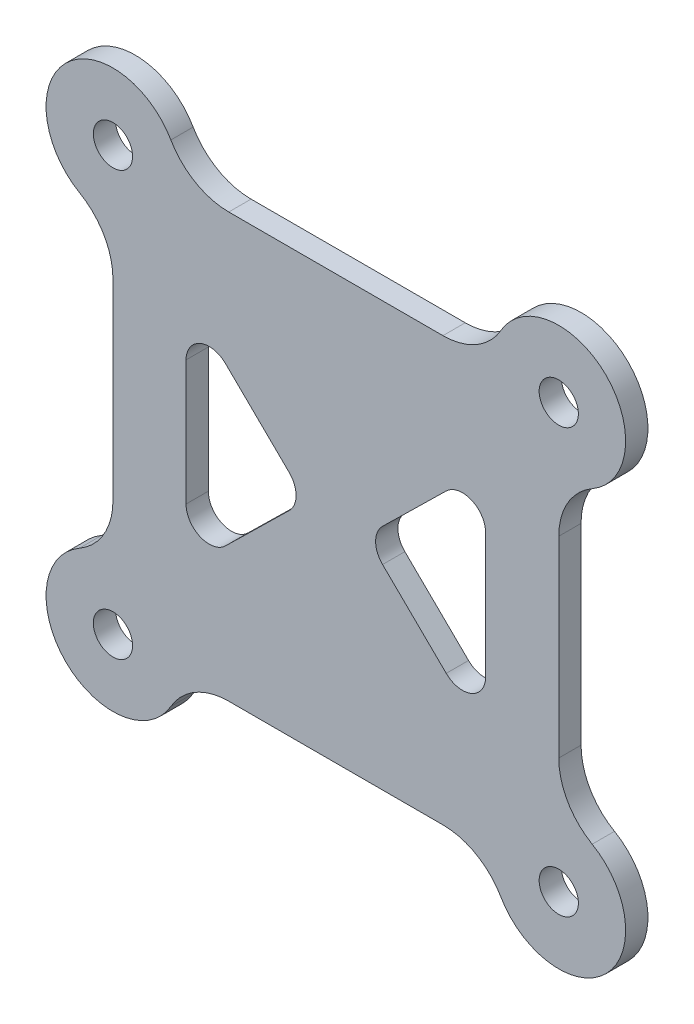
ISO-10303-21;
HEADER;
FILE_DESCRIPTION(('STEP AP214'),'2;1');
FILE_NAME('part.step','',(''),(''),'','','');
FILE_SCHEMA(('AUTOMOTIVE_DESIGN { 1 0 10303 214 1 1 1 1 }'));
ENDSEC;
DATA;
#1=APPLICATION_CONTEXT('core data for automotive mechanical design processes');
#2=APPLICATION_PROTOCOL_DEFINITION('international standard','automotive_design',2000,#1);
#3=PRODUCT_CONTEXT('',#1,'mechanical');
#4=PRODUCT('Part','Part','',(#3));
#5=PRODUCT_RELATED_PRODUCT_CATEGORY('part','',(#4));
#6=PRODUCT_DEFINITION_FORMATION('','',#4);
#7=PRODUCT_DEFINITION_CONTEXT('part definition',#1,'design');
#8=PRODUCT_DEFINITION('design','',#6,#7);
#9=PRODUCT_DEFINITION_SHAPE('','',#8);
#10=(LENGTH_UNIT() NAMED_UNIT(*) SI_UNIT(.MILLI.,.METRE.));
#11=(NAMED_UNIT(*) PLANE_ANGLE_UNIT() SI_UNIT($,.RADIAN.));
#12=(NAMED_UNIT(*) SI_UNIT($,.STERADIAN.) SOLID_ANGLE_UNIT());
#13=UNCERTAINTY_MEASURE_WITH_UNIT(LENGTH_MEASURE(1.E-05),#10,'distance_accuracy_value','');
#14=(GEOMETRIC_REPRESENTATION_CONTEXT(3) GLOBAL_UNCERTAINTY_ASSIGNED_CONTEXT((#13)) GLOBAL_UNIT_ASSIGNED_CONTEXT((#10,
#11,#12)) REPRESENTATION_CONTEXT('',''));
#15=CARTESIAN_POINT('',(0.,0.,0.));
#16=DIRECTION('',(0.,0.,1.));
#17=DIRECTION('',(1.,0.,0.));
#18=AXIS2_PLACEMENT_3D('',#15,#16,#17);
#19=CARTESIAN_POINT('',(-0.600480947161671,1.563,0.125));
#20=DIRECTION('',(0.,0.,1.));
#21=DIRECTION('',(1.,0.,0.));
#22=AXIS2_PLACEMENT_3D('',#19,#20,#21);
#23=PLANE('',#22);
#24=CARTESIAN_POINT('',(1.25,-1.188,0.125));
#25=DIRECTION('',(0.,0.,1.));
#26=DIRECTION('',(1.,0.,0.));
#27=AXIS2_PLACEMENT_3D('',#24,#25,#26);
#28=CIRCLE('',#27,0.11);
#29=CARTESIAN_POINT('',(1.36,-1.188,0.125));
#30=VERTEX_POINT('',#29);
#31=EDGE_CURVE('E929',#30,#30,#28,.F.);
#32=ORIENTED_EDGE('',*,*,#31,.T.);
#33=EDGE_LOOP('',(#32));
#34=FACE_BOUND('',#33,.T.);
#35=CARTESIAN_POINT('',(-1.25,-1.188,0.125));
#36=DIRECTION('',(0.,0.,1.));
#37=DIRECTION('',(1.,0.,0.));
#38=AXIS2_PLACEMENT_3D('',#35,#36,#37);
#39=CIRCLE('',#38,0.11);
#40=CARTESIAN_POINT('',(-1.14,-1.188,0.125));
#41=VERTEX_POINT('',#40);
#42=EDGE_CURVE('E940',#41,#41,#39,.F.);
#43=ORIENTED_EDGE('',*,*,#42,.T.);
#44=EDGE_LOOP('',(#43));
#45=FACE_BOUND('',#44,.T.);
#46=CARTESIAN_POINT('',(1.25,1.188,0.125));
#47=DIRECTION('',(0.,0.,1.));
#48=DIRECTION('',(1.,0.,0.));
#49=AXIS2_PLACEMENT_3D('',#46,#47,#48);
#50=CIRCLE('',#49,0.11);
#51=CARTESIAN_POINT('',(1.36,1.188,0.125));
#52=VERTEX_POINT('',#51);
#53=EDGE_CURVE('E594',#52,#52,#50,.T.);
#54=ORIENTED_EDGE('',*,*,#53,.F.);
#55=EDGE_LOOP('',(#54));
#56=FACE_BOUND('',#55,.T.);
#57=DIRECTION('',(0.714142842854285,0.7,0.));
#58=VECTOR('',#57,1.);
#59=CARTESIAN_POINT('',(0.0819350035006998,-0.0835904233275223,0.125));
#60=LINE('',#59,#58);
#61=CARTESIAN_POINT('',(0.261928578572857,0.0928385695710571,0.125));
#62=VERTEX_POINT('',#61);
#63=CARTESIAN_POINT('',(0.619,0.442838569571057,0.125));
#64=VERTEX_POINT('',#63);
#65=EDGE_CURVE('E572',#62,#64,#60,.T.);
#66=ORIENTED_EDGE('',*,*,#65,.T.);
#67=CARTESIAN_POINT('',(0.709999999999999,0.35,0.125));
#68=DIRECTION('',(0.,0.,1.));
#69=DIRECTION('',(1.,0.,0.));
#70=AXIS2_PLACEMENT_3D('',#67,#68,#69);
#71=CIRCLE('',#70,0.13);
#72=CARTESIAN_POINT('',(0.839999999999999,0.35,0.125));
#73=VERTEX_POINT('',#72);
#74=EDGE_CURVE('E595',#64,#73,#71,.F.);
#75=ORIENTED_EDGE('',*,*,#74,.T.);
#76=DIRECTION('',(0.,-1.,0.));
#77=VECTOR('',#76,1.);
#78=CARTESIAN_POINT('',(0.84,0.,0.125));
#79=LINE('',#78,#77);
#80=CARTESIAN_POINT('',(0.84,-0.35,0.125));
#81=VERTEX_POINT('',#80);
#82=EDGE_CURVE('E392',#73,#81,#79,.T.);
#83=ORIENTED_EDGE('',*,*,#82,.T.);
#84=CARTESIAN_POINT('',(0.71,-0.35,0.125));
#85=DIRECTION('',(0.,0.,1.));
#86=DIRECTION('',(1.,0.,0.));
#87=AXIS2_PLACEMENT_3D('',#84,#85,#86);
#88=CIRCLE('',#87,0.13);
#89=CARTESIAN_POINT('',(0.618999999999999,-0.442838569571057,0.125));
#90=VERTEX_POINT('',#89);
#91=EDGE_CURVE('E586',#81,#90,#88,.F.);
#92=ORIENTED_EDGE('',*,*,#91,.T.);
#93=DIRECTION('',(-0.714142842854285,0.7,0.));
#94=VECTOR('',#93,1.);
#95=CARTESIAN_POINT('',(0.0819350035007,0.0835904233275223,0.125));
#96=LINE('',#95,#94);
#97=CARTESIAN_POINT('',(0.261928578572857,-0.0928385695710571,0.125));
#98=VERTEX_POINT('',#97);
#99=EDGE_CURVE('E582',#90,#98,#96,.T.);
#100=ORIENTED_EDGE('',*,*,#99,.T.);
#101=CARTESIAN_POINT('',(0.352928578572857,0.,0.125));
#102=DIRECTION('',(0.,0.,1.));
#103=DIRECTION('',(1.,0.,0.));
#104=AXIS2_PLACEMENT_3D('',#101,#102,#103);
#105=CIRCLE('',#104,0.13);
#106=EDGE_CURVE('E564',#62,#98,#105,.T.);
#107=ORIENTED_EDGE('',*,*,#106,.F.);
#108=EDGE_LOOP('',(#66,#75,#83,#92,#100,#107));
#109=FACE_BOUND('',#108,.T.);
#110=CARTESIAN_POINT('',(-0.352928578572857,0.,0.125));
#111=DIRECTION('',(0.,0.,1.));
#112=DIRECTION('',(1.,0.,0.));
#113=AXIS2_PLACEMENT_3D('',#110,#111,#112);
#114=CIRCLE('',#113,0.13);
#115=CARTESIAN_POINT('',(-0.261928578572857,0.0928385695710571,0.125));
#116=VERTEX_POINT('',#115);
#117=CARTESIAN_POINT('',(-0.261928578572857,-0.0928385695710571,0.125));
#118=VERTEX_POINT('',#117);
#119=EDGE_CURVE('E618',#116,#118,#114,.F.);
#120=ORIENTED_EDGE('',*,*,#119,.T.);
#121=DIRECTION('',(0.714142842854285,0.7,0.));
#122=VECTOR('',#121,1.);
#123=CARTESIAN_POINT('',(-0.0819350035007,0.0835904233275223,0.125));
#124=LINE('',#123,#122);
#125=CARTESIAN_POINT('',(-0.618999999999999,-0.442838569571057,0.125));
#126=VERTEX_POINT('',#125);
#127=EDGE_CURVE('E627',#126,#118,#124,.T.);
#128=ORIENTED_EDGE('',*,*,#127,.F.);
#129=CARTESIAN_POINT('',(-0.71,-0.35,0.125));
#130=DIRECTION('',(0.,0.,1.));
#131=DIRECTION('',(1.,0.,0.));
#132=AXIS2_PLACEMENT_3D('',#129,#130,#131);
#133=CIRCLE('',#132,0.13);
#134=CARTESIAN_POINT('',(-0.84,-0.35,0.125));
#135=VERTEX_POINT('',#134);
#136=EDGE_CURVE('E626',#135,#126,#133,.T.);
#137=ORIENTED_EDGE('',*,*,#136,.F.);
#138=DIRECTION('',(0.,-1.,0.));
#139=VECTOR('',#138,1.);
#140=CARTESIAN_POINT('',(-0.84,0.,0.125));
#141=LINE('',#140,#139);
#142=CARTESIAN_POINT('',(-0.84,0.35,0.125));
#143=VERTEX_POINT('',#142);
#144=EDGE_CURVE('E624',#143,#135,#141,.T.);
#145=ORIENTED_EDGE('',*,*,#144,.F.);
#146=CARTESIAN_POINT('',(-0.709999999999999,0.35,0.125));
#147=DIRECTION('',(0.,0.,1.));
#148=DIRECTION('',(1.,0.,0.));
#149=AXIS2_PLACEMENT_3D('',#146,#147,#148);
#150=CIRCLE('',#149,0.13);
#151=CARTESIAN_POINT('',(-0.619,0.442838569571057,0.125));
#152=VERTEX_POINT('',#151);
#153=EDGE_CURVE('E625',#152,#143,#150,.T.);
#154=ORIENTED_EDGE('',*,*,#153,.F.);
#155=DIRECTION('',(-0.714142842854285,0.7,0.));
#156=VECTOR('',#155,1.);
#157=CARTESIAN_POINT('',(-0.0819350035006998,-0.0835904233275223,0.125));
#158=LINE('',#157,#156);
#159=EDGE_CURVE('E620',#116,#152,#158,.T.);
#160=ORIENTED_EDGE('',*,*,#159,.F.);
#161=EDGE_LOOP('',(#120,#128,#137,#145,#154,#160));
#162=FACE_BOUND('',#161,.T.);
#163=CARTESIAN_POINT('',(-0.600480947161671,1.563,0.125));
#164=DIRECTION('',(0.,0.,1.));
#165=DIRECTION('',(1.,0.,0.));
#166=AXIS2_PLACEMENT_3D('',#163,#164,#165);
#167=CIRCLE('',#166,0.375);
#168=CARTESIAN_POINT('',(-0.925240473580835,1.3755,0.125));
#169=VERTEX_POINT('',#168);
#170=CARTESIAN_POINT('',(-0.600480947161671,1.188,0.125));
#171=VERTEX_POINT('',#170);
#172=EDGE_CURVE('E656',#169,#171,#167,.T.);
#173=ORIENTED_EDGE('',*,*,#172,.F.);
#174=CARTESIAN_POINT('',(-1.25,1.188,0.125));
#175=DIRECTION('',(0.,0.,1.));
#176=DIRECTION('',(1.,0.,0.));
#177=AXIS2_PLACEMENT_3D('',#174,#175,#176);
#178=CIRCLE('',#177,0.375);
#179=CARTESIAN_POINT('',(-1.4375,0.863240473580835,0.125));
#180=VERTEX_POINT('',#179);
#181=EDGE_CURVE('E699',#169,#180,#178,.T.);
#182=ORIENTED_EDGE('',*,*,#181,.T.);
#183=CARTESIAN_POINT('',(-1.625,0.53848094716167,0.125));
#184=DIRECTION('',(0.,0.,1.));
#185=DIRECTION('',(1.,0.,0.));
#186=AXIS2_PLACEMENT_3D('',#183,#184,#185);
#187=CIRCLE('',#186,0.375);
#188=CARTESIAN_POINT('',(-1.25,0.53848094716167,0.125));
#189=VERTEX_POINT('',#188);
#190=EDGE_CURVE('E697',#189,#180,#187,.T.);
#191=ORIENTED_EDGE('',*,*,#190,.F.);
#192=DIRECTION('',(0.,-1.,0.));
#193=VECTOR('',#192,1.);
#194=CARTESIAN_POINT('',(-1.25,0.53848094716167,0.125));
#195=LINE('',#194,#193);
#196=CARTESIAN_POINT('',(-1.25,-0.538480947161671,0.125));
#197=VERTEX_POINT('',#196);
#198=EDGE_CURVE('E694',#189,#197,#195,.T.);
#199=ORIENTED_EDGE('',*,*,#198,.T.);
#200=CARTESIAN_POINT('',(-1.625,-0.53848094716167,0.125));
#201=DIRECTION('',(0.,0.,-1.));
#202=DIRECTION('',(-1.,0.,0.));
#203=AXIS2_PLACEMENT_3D('',#200,#201,#202);
#204=CIRCLE('',#203,0.375);
#205=CARTESIAN_POINT('',(-1.4375,-0.863240473580835,0.125));
#206=VERTEX_POINT('',#205);
#207=EDGE_CURVE('E695',#197,#206,#204,.T.);
#208=ORIENTED_EDGE('',*,*,#207,.T.);
#209=CARTESIAN_POINT('',(-1.25,-1.188,0.125));
#210=DIRECTION('',(0.,0.,-1.));
#211=DIRECTION('',(-1.,0.,0.));
#212=AXIS2_PLACEMENT_3D('',#209,#210,#211);
#213=CIRCLE('',#212,0.375);
#214=CARTESIAN_POINT('',(-0.925240473580835,-1.3755,0.125));
#215=VERTEX_POINT('',#214);
#216=EDGE_CURVE('E686',#215,#206,#213,.T.);
#217=ORIENTED_EDGE('',*,*,#216,.F.);
#218=CARTESIAN_POINT('',(-0.600480947161671,-1.563,0.125));
#219=DIRECTION('',(0.,0.,-1.));
#220=DIRECTION('',(-1.,0.,0.));
#221=AXIS2_PLACEMENT_3D('',#218,#219,#220);
#222=CIRCLE('',#221,0.375);
#223=CARTESIAN_POINT('',(-0.600480947161671,-1.188,0.125));
#224=VERTEX_POINT('',#223);
#225=EDGE_CURVE('E690',#215,#224,#222,.T.);
#226=ORIENTED_EDGE('',*,*,#225,.T.);
#227=DIRECTION('',(1.,0.,0.));
#228=VECTOR('',#227,1.);
#229=CARTESIAN_POINT('',(-0.600480947161671,-1.188,0.125));
#230=LINE('',#229,#228);
#231=CARTESIAN_POINT('',(0.600480947161671,-1.188,0.125));
#232=VERTEX_POINT('',#231);
#233=EDGE_CURVE('E684',#224,#232,#230,.T.);
#234=ORIENTED_EDGE('',*,*,#233,.T.);
#235=CARTESIAN_POINT('',(0.600480947161671,-1.563,0.125));
#236=DIRECTION('',(0.,0.,1.));
#237=DIRECTION('',(1.,0.,0.));
#238=AXIS2_PLACEMENT_3D('',#235,#236,#237);
#239=CIRCLE('',#238,0.375);
#240=CARTESIAN_POINT('',(0.925240473580835,-1.3755,0.125));
#241=VERTEX_POINT('',#240);
#242=EDGE_CURVE('E685',#241,#232,#239,.T.);
#243=ORIENTED_EDGE('',*,*,#242,.F.);
#244=CARTESIAN_POINT('',(1.25,-1.188,0.125));
#245=DIRECTION('',(0.,0.,-1.));
#246=DIRECTION('',(-1.,0.,0.));
#247=AXIS2_PLACEMENT_3D('',#244,#245,#246);
#248=CIRCLE('',#247,0.375);
#249=CARTESIAN_POINT('',(1.4375,-0.863240473580835,0.125));
#250=VERTEX_POINT('',#249);
#251=EDGE_CURVE('E677',#250,#241,#248,.T.);
#252=ORIENTED_EDGE('',*,*,#251,.F.);
#253=CARTESIAN_POINT('',(1.625,-0.538480947161671,0.125));
#254=DIRECTION('',(0.,0.,1.));
#255=DIRECTION('',(1.,0.,0.));
#256=AXIS2_PLACEMENT_3D('',#253,#254,#255);
#257=CIRCLE('',#256,0.375);
#258=CARTESIAN_POINT('',(1.25,-0.538480947161671,0.125));
#259=VERTEX_POINT('',#258);
#260=EDGE_CURVE('E676',#259,#250,#257,.T.);
#261=ORIENTED_EDGE('',*,*,#260,.F.);
#262=DIRECTION('',(0.,-1.,0.));
#263=VECTOR('',#262,1.);
#264=CARTESIAN_POINT('',(1.25,0.538480947161671,0.125));
#265=LINE('',#264,#263);
#266=CARTESIAN_POINT('',(1.25,0.538480947161671,0.125));
#267=VERTEX_POINT('',#266);
#268=EDGE_CURVE('E673',#267,#259,#265,.T.);
#269=ORIENTED_EDGE('',*,*,#268,.F.);
#270=CARTESIAN_POINT('',(1.625,0.538480947161671,0.125));
#271=DIRECTION('',(0.,0.,-1.));
#272=DIRECTION('',(-1.,0.,0.));
#273=AXIS2_PLACEMENT_3D('',#270,#271,#272);
#274=CIRCLE('',#273,0.375);
#275=CARTESIAN_POINT('',(1.4375,0.863240473580835,0.125));
#276=VERTEX_POINT('',#275);
#277=EDGE_CURVE('E671',#267,#276,#274,.T.);
#278=ORIENTED_EDGE('',*,*,#277,.T.);
#279=CARTESIAN_POINT('',(1.25,1.188,0.125));
#280=DIRECTION('',(0.,0.,1.));
#281=DIRECTION('',(1.,0.,0.));
#282=AXIS2_PLACEMENT_3D('',#279,#280,#281);
#283=CIRCLE('',#282,0.375);
#284=CARTESIAN_POINT('',(0.925240473580835,1.3755,0.125));
#285=VERTEX_POINT('',#284);
#286=EDGE_CURVE('E669',#276,#285,#283,.T.);
#287=ORIENTED_EDGE('',*,*,#286,.T.);
#288=CARTESIAN_POINT('',(0.600480947161671,1.563,0.125));
#289=DIRECTION('',(0.,0.,-1.));
#290=DIRECTION('',(-1.,0.,0.));
#291=AXIS2_PLACEMENT_3D('',#288,#289,#290);
#292=CIRCLE('',#291,0.375);
#293=CARTESIAN_POINT('',(0.600480947161671,1.188,0.125));
#294=VERTEX_POINT('',#293);
#295=EDGE_CURVE('E670',#285,#294,#292,.T.);
#296=ORIENTED_EDGE('',*,*,#295,.T.);
#297=DIRECTION('',(1.,0.,0.));
#298=VECTOR('',#297,1.);
#299=CARTESIAN_POINT('',(-0.600480947161671,1.188,0.125));
#300=LINE('',#299,#298);
#301=EDGE_CURVE('E661',#171,#294,#300,.T.);
#302=ORIENTED_EDGE('',*,*,#301,.F.);
#303=EDGE_LOOP('',(#173,#182,#191,#199,#208,#217,#226,#234,#243,#252,#261,#269,#278,#287,#296,#302));
#304=FACE_BOUND('',#303,.T.);
#305=CARTESIAN_POINT('',(-1.25,1.188,0.125));
#306=DIRECTION('',(0.,0.,1.));
#307=DIRECTION('',(1.,0.,0.));
#308=AXIS2_PLACEMENT_3D('',#305,#306,#307);
#309=CIRCLE('',#308,0.11);
#310=CARTESIAN_POINT('',(-1.14,1.188,0.125));
#311=VERTEX_POINT('',#310);
#312=EDGE_CURVE('E943',#311,#311,#309,.T.);
#313=ORIENTED_EDGE('',*,*,#312,.F.);
#314=EDGE_LOOP('',(#313));
#315=FACE_BOUND('',#314,.T.);
#316=ADVANCED_FACE('F373',(#34,#45,#56,#109,#162,#304,#315),#23,.T.);
#317=CARTESIAN_POINT('',(-0.600480947161671,1.563,0.));
#318=DIRECTION('',(0.,0.,1.));
#319=DIRECTION('',(1.,0.,0.));
#320=AXIS2_PLACEMENT_3D('',#317,#318,#319);
#321=PLANE('',#320);
#322=CARTESIAN_POINT('',(1.25,-1.188,0.));
#323=DIRECTION('',(0.,0.,1.));
#324=DIRECTION('',(1.,0.,0.));
#325=AXIS2_PLACEMENT_3D('',#322,#323,#324);
#326=CIRCLE('',#325,0.11);
#327=CARTESIAN_POINT('',(1.36,-1.188,0.));
#328=VERTEX_POINT('',#327);
#329=EDGE_CURVE('E932',#328,#328,#326,.F.);
#330=ORIENTED_EDGE('',*,*,#329,.F.);
#331=EDGE_LOOP('',(#330));
#332=FACE_BOUND('',#331,.T.);
#333=CARTESIAN_POINT('',(-1.25,-1.188,0.));
#334=DIRECTION('',(0.,0.,1.));
#335=DIRECTION('',(1.,0.,0.));
#336=AXIS2_PLACEMENT_3D('',#333,#334,#335);
#337=CIRCLE('',#336,0.11);
#338=CARTESIAN_POINT('',(-1.14,-1.188,0.));
#339=VERTEX_POINT('',#338);
#340=EDGE_CURVE('E935',#339,#339,#337,.F.);
#341=ORIENTED_EDGE('',*,*,#340,.F.);
#342=EDGE_LOOP('',(#341));
#343=FACE_BOUND('',#342,.T.);
#344=CARTESIAN_POINT('',(0.709999999999999,0.35,0.));
#345=DIRECTION('',(0.,0.,1.));
#346=DIRECTION('',(1.,0.,0.));
#347=AXIS2_PLACEMENT_3D('',#344,#345,#346);
#348=CIRCLE('',#347,0.13);
#349=CARTESIAN_POINT('',(0.618999999999999,0.442838569571057,0.));
#350=VERTEX_POINT('',#349);
#351=CARTESIAN_POINT('',(0.84,0.35,0.));
#352=VERTEX_POINT('',#351);
#353=EDGE_CURVE('E576',#350,#352,#348,.F.);
#354=ORIENTED_EDGE('',*,*,#353,.F.);
#355=DIRECTION('',(0.714142842854285,0.7,0.));
#356=VECTOR('',#355,1.);
#357=CARTESIAN_POINT('',(0.0819350035006998,-0.0835904233275223,0.));
#358=LINE('',#357,#356);
#359=CARTESIAN_POINT('',(0.261928578572857,0.0928385695710571,0.));
#360=VERTEX_POINT('',#359);
#361=EDGE_CURVE('E397',#360,#350,#358,.T.);
#362=ORIENTED_EDGE('',*,*,#361,.F.);
#363=CARTESIAN_POINT('',(0.352928578572857,0.,0.));
#364=DIRECTION('',(0.,0.,1.));
#365=DIRECTION('',(1.,0.,0.));
#366=AXIS2_PLACEMENT_3D('',#363,#364,#365);
#367=CIRCLE('',#366,0.13);
#368=CARTESIAN_POINT('',(0.261928578572857,-0.0928385695710571,0.));
#369=VERTEX_POINT('',#368);
#370=EDGE_CURVE('E570',#360,#369,#367,.T.);
#371=ORIENTED_EDGE('',*,*,#370,.T.);
#372=DIRECTION('',(-0.714142842854285,0.7,0.));
#373=VECTOR('',#372,1.);
#374=CARTESIAN_POINT('',(0.0819350035007,0.0835904233275223,0.));
#375=LINE('',#374,#373);
#376=CARTESIAN_POINT('',(0.618999999999999,-0.442838569571057,0.));
#377=VERTEX_POINT('',#376);
#378=EDGE_CURVE('E600',#377,#369,#375,.T.);
#379=ORIENTED_EDGE('',*,*,#378,.F.);
#380=CARTESIAN_POINT('',(0.71,-0.35,0.));
#381=DIRECTION('',(0.,0.,1.));
#382=DIRECTION('',(1.,0.,0.));
#383=AXIS2_PLACEMENT_3D('',#380,#381,#382);
#384=CIRCLE('',#383,0.13);
#385=CARTESIAN_POINT('',(0.84,-0.35,0.));
#386=VERTEX_POINT('',#385);
#387=EDGE_CURVE('E598',#386,#377,#384,.F.);
#388=ORIENTED_EDGE('',*,*,#387,.F.);
#389=DIRECTION('',(0.,-1.,0.));
#390=VECTOR('',#389,1.);
#391=CARTESIAN_POINT('',(0.84,0.,0.));
#392=LINE('',#391,#390);
#393=EDGE_CURVE('E603',#352,#386,#392,.T.);
#394=ORIENTED_EDGE('',*,*,#393,.F.);
#395=EDGE_LOOP('',(#354,#362,#371,#379,#388,#394));
#396=FACE_BOUND('',#395,.T.);
#397=DIRECTION('',(0.714142842854285,0.7,0.));
#398=VECTOR('',#397,1.);
#399=CARTESIAN_POINT('',(-0.0819350035007,0.0835904233275223,0.));
#400=LINE('',#399,#398);
#401=CARTESIAN_POINT('',(-0.618999999999999,-0.442838569571057,0.));
#402=VERTEX_POINT('',#401);
#403=CARTESIAN_POINT('',(-0.261928578572857,-0.0928385695710573,0.));
#404=VERTEX_POINT('',#403);
#405=EDGE_CURVE('E619',#402,#404,#400,.T.);
#406=ORIENTED_EDGE('',*,*,#405,.T.);
#407=CARTESIAN_POINT('',(-0.352928578572857,0.,0.));
#408=DIRECTION('',(0.,0.,1.));
#409=DIRECTION('',(1.,0.,0.));
#410=AXIS2_PLACEMENT_3D('',#407,#408,#409);
#411=CIRCLE('',#410,0.13);
#412=CARTESIAN_POINT('',(-0.261928578572857,0.0928385695710571,0.));
#413=VERTEX_POINT('',#412);
#414=EDGE_CURVE('E568',#413,#404,#411,.F.);
#415=ORIENTED_EDGE('',*,*,#414,.F.);
#416=DIRECTION('',(-0.714142842854285,0.7,0.));
#417=VECTOR('',#416,1.);
#418=CARTESIAN_POINT('',(-0.0819350035006998,-0.0835904233275223,0.));
#419=LINE('',#418,#417);
#420=CARTESIAN_POINT('',(-0.619,0.442838569571057,0.));
#421=VERTEX_POINT('',#420);
#422=EDGE_CURVE('E633',#413,#421,#419,.T.);
#423=ORIENTED_EDGE('',*,*,#422,.T.);
#424=CARTESIAN_POINT('',(-0.709999999999999,0.35,0.));
#425=DIRECTION('',(0.,0.,1.));
#426=DIRECTION('',(1.,0.,0.));
#427=AXIS2_PLACEMENT_3D('',#424,#425,#426);
#428=CIRCLE('',#427,0.13);
#429=CARTESIAN_POINT('',(-0.84,0.35,0.));
#430=VERTEX_POINT('',#429);
#431=EDGE_CURVE('E636',#421,#430,#428,.T.);
#432=ORIENTED_EDGE('',*,*,#431,.T.);
#433=DIRECTION('',(0.,-1.,0.));
#434=VECTOR('',#433,1.);
#435=CARTESIAN_POINT('',(-0.84,0.,0.));
#436=LINE('',#435,#434);
#437=CARTESIAN_POINT('',(-0.84,-0.35,0.));
#438=VERTEX_POINT('',#437);
#439=EDGE_CURVE('E638',#430,#438,#436,.T.);
#440=ORIENTED_EDGE('',*,*,#439,.T.);
#441=CARTESIAN_POINT('',(-0.71,-0.35,0.));
#442=DIRECTION('',(0.,0.,1.));
#443=DIRECTION('',(1.,0.,0.));
#444=AXIS2_PLACEMENT_3D('',#441,#442,#443);
#445=CIRCLE('',#444,0.13);
#446=EDGE_CURVE('E645',#438,#402,#445,.T.);
#447=ORIENTED_EDGE('',*,*,#446,.T.);
#448=EDGE_LOOP('',(#406,#415,#423,#432,#440,#447));
#449=FACE_BOUND('',#448,.T.);
#450=CARTESIAN_POINT('',(-0.600480947161671,1.563,0.));
#451=DIRECTION('',(0.,0.,1.));
#452=DIRECTION('',(1.,0.,0.));
#453=AXIS2_PLACEMENT_3D('',#450,#451,#452);
#454=CIRCLE('',#453,0.375);
#455=CARTESIAN_POINT('',(-0.925240473580835,1.3755,0.));
#456=VERTEX_POINT('',#455);
#457=CARTESIAN_POINT('',(-0.600480947161671,1.188,0.));
#458=VERTEX_POINT('',#457);
#459=EDGE_CURVE('E659',#456,#458,#454,.T.);
#460=ORIENTED_EDGE('',*,*,#459,.T.);
#461=DIRECTION('',(1.,0.,0.));
#462=VECTOR('',#461,1.);
#463=CARTESIAN_POINT('',(-0.600480947161671,1.188,0.));
#464=LINE('',#463,#462);
#465=CARTESIAN_POINT('',(0.600480947161671,1.188,0.));
#466=VERTEX_POINT('',#465);
#467=EDGE_CURVE('E703',#458,#466,#464,.T.);
#468=ORIENTED_EDGE('',*,*,#467,.T.);
#469=CARTESIAN_POINT('',(0.600480947161671,1.563,0.));
#470=DIRECTION('',(0.,0.,-1.));
#471=DIRECTION('',(-1.,0.,0.));
#472=AXIS2_PLACEMENT_3D('',#469,#470,#471);
#473=CIRCLE('',#472,0.375);
#474=CARTESIAN_POINT('',(0.925240473580835,1.3755,0.));
#475=VERTEX_POINT('',#474);
#476=EDGE_CURVE('E708',#475,#466,#473,.T.);
#477=ORIENTED_EDGE('',*,*,#476,.F.);
#478=CARTESIAN_POINT('',(1.25,1.188,0.));
#479=DIRECTION('',(0.,0.,1.));
#480=DIRECTION('',(1.,0.,0.));
#481=AXIS2_PLACEMENT_3D('',#478,#479,#480);
#482=CIRCLE('',#481,0.375);
#483=CARTESIAN_POINT('',(1.4375,0.863240473580835,0.));
#484=VERTEX_POINT('',#483);
#485=EDGE_CURVE('E710',#484,#475,#482,.T.);
#486=ORIENTED_EDGE('',*,*,#485,.F.);
#487=CARTESIAN_POINT('',(1.625,0.538480947161671,0.));
#488=DIRECTION('',(0.,0.,-1.));
#489=DIRECTION('',(-1.,0.,0.));
#490=AXIS2_PLACEMENT_3D('',#487,#488,#489);
#491=CIRCLE('',#490,0.375);
#492=CARTESIAN_POINT('',(1.25,0.538480947161671,0.));
#493=VERTEX_POINT('',#492);
#494=EDGE_CURVE('E713',#493,#484,#491,.T.);
#495=ORIENTED_EDGE('',*,*,#494,.F.);
#496=DIRECTION('',(0.,-1.,0.));
#497=VECTOR('',#496,1.);
#498=CARTESIAN_POINT('',(1.25,0.538480947161671,0.));
#499=LINE('',#498,#497);
#500=CARTESIAN_POINT('',(1.25,-0.538480947161671,0.));
#501=VERTEX_POINT('',#500);
#502=EDGE_CURVE('E711',#493,#501,#499,.T.);
#503=ORIENTED_EDGE('',*,*,#502,.T.);
#504=CARTESIAN_POINT('',(1.625,-0.538480947161671,0.));
#505=DIRECTION('',(0.,0.,1.));
#506=DIRECTION('',(1.,0.,0.));
#507=AXIS2_PLACEMENT_3D('',#504,#505,#506);
#508=CIRCLE('',#507,0.375);
#509=CARTESIAN_POINT('',(1.4375,-0.863240473580835,0.));
#510=VERTEX_POINT('',#509);
#511=EDGE_CURVE('E716',#501,#510,#508,.T.);
#512=ORIENTED_EDGE('',*,*,#511,.T.);
#513=CARTESIAN_POINT('',(1.25,-1.188,0.));
#514=DIRECTION('',(0.,0.,-1.));
#515=DIRECTION('',(-1.,0.,0.));
#516=AXIS2_PLACEMENT_3D('',#513,#514,#515);
#517=CIRCLE('',#516,0.375);
#518=CARTESIAN_POINT('',(0.925240473580835,-1.3755,0.));
#519=VERTEX_POINT('',#518);
#520=EDGE_CURVE('E717',#510,#519,#517,.T.);
#521=ORIENTED_EDGE('',*,*,#520,.T.);
#522=CARTESIAN_POINT('',(0.600480947161671,-1.563,0.));
#523=DIRECTION('',(0.,0.,1.));
#524=DIRECTION('',(1.,0.,0.));
#525=AXIS2_PLACEMENT_3D('',#522,#523,#524);
#526=CIRCLE('',#525,0.375);
#527=CARTESIAN_POINT('',(0.600480947161671,-1.188,0.));
#528=VERTEX_POINT('',#527);
#529=EDGE_CURVE('E725',#519,#528,#526,.T.);
#530=ORIENTED_EDGE('',*,*,#529,.T.);
#531=DIRECTION('',(1.,0.,0.));
#532=VECTOR('',#531,1.);
#533=CARTESIAN_POINT('',(-0.600480947161671,-1.188,0.));
#534=LINE('',#533,#532);
#535=CARTESIAN_POINT('',(-0.600480947161671,-1.188,0.));
#536=VERTEX_POINT('',#535);
#537=EDGE_CURVE('E724',#536,#528,#534,.T.);
#538=ORIENTED_EDGE('',*,*,#537,.F.);
#539=CARTESIAN_POINT('',(-0.600480947161671,-1.563,0.));
#540=DIRECTION('',(0.,0.,-1.));
#541=DIRECTION('',(-1.,0.,0.));
#542=AXIS2_PLACEMENT_3D('',#539,#540,#541);
#543=CIRCLE('',#542,0.375);
#544=CARTESIAN_POINT('',(-0.925240473580835,-1.3755,0.));
#545=VERTEX_POINT('',#544);
#546=EDGE_CURVE('E727',#545,#536,#543,.T.);
#547=ORIENTED_EDGE('',*,*,#546,.F.);
#548=CARTESIAN_POINT('',(-1.25,-1.188,0.));
#549=DIRECTION('',(0.,0.,-1.));
#550=DIRECTION('',(-1.,0.,0.));
#551=AXIS2_PLACEMENT_3D('',#548,#549,#550);
#552=CIRCLE('',#551,0.375);
#553=CARTESIAN_POINT('',(-1.4375,-0.863240473580835,0.));
#554=VERTEX_POINT('',#553);
#555=EDGE_CURVE('E729',#545,#554,#552,.T.);
#556=ORIENTED_EDGE('',*,*,#555,.T.);
#557=CARTESIAN_POINT('',(-1.625,-0.53848094716167,0.));
#558=DIRECTION('',(0.,0.,-1.));
#559=DIRECTION('',(-1.,0.,0.));
#560=AXIS2_PLACEMENT_3D('',#557,#558,#559);
#561=CIRCLE('',#560,0.375);
#562=CARTESIAN_POINT('',(-1.25,-0.538480947161671,0.));
#563=VERTEX_POINT('',#562);
#564=EDGE_CURVE('E734',#563,#554,#561,.T.);
#565=ORIENTED_EDGE('',*,*,#564,.F.);
#566=DIRECTION('',(0.,-1.,0.));
#567=VECTOR('',#566,1.);
#568=CARTESIAN_POINT('',(-1.25,0.53848094716167,0.));
#569=LINE('',#568,#567);
#570=CARTESIAN_POINT('',(-1.25,0.53848094716167,0.));
#571=VERTEX_POINT('',#570);
#572=EDGE_CURVE('E737',#571,#563,#569,.T.);
#573=ORIENTED_EDGE('',*,*,#572,.F.);
#574=CARTESIAN_POINT('',(-1.625,0.53848094716167,0.));
#575=DIRECTION('',(0.,0.,1.));
#576=DIRECTION('',(1.,0.,0.));
#577=AXIS2_PLACEMENT_3D('',#574,#575,#576);
#578=CIRCLE('',#577,0.375);
#579=CARTESIAN_POINT('',(-1.4375,0.863240473580835,0.));
#580=VERTEX_POINT('',#579);
#581=EDGE_CURVE('E738',#571,#580,#578,.T.);
#582=ORIENTED_EDGE('',*,*,#581,.T.);
#583=CARTESIAN_POINT('',(-1.25,1.188,0.));
#584=DIRECTION('',(0.,0.,1.));
#585=DIRECTION('',(1.,0.,0.));
#586=AXIS2_PLACEMENT_3D('',#583,#584,#585);
#587=CIRCLE('',#586,0.375);
#588=EDGE_CURVE('E665',#456,#580,#587,.T.);
#589=ORIENTED_EDGE('',*,*,#588,.F.);
#590=EDGE_LOOP('',(#460,#468,#477,#486,#495,#503,#512,#521,#530,#538,#547,#556,#565,#573,#582,#589));
#591=FACE_BOUND('',#590,.T.);
#592=CARTESIAN_POINT('',(1.25,1.188,0.));
#593=DIRECTION('',(0.,0.,1.));
#594=DIRECTION('',(1.,0.,0.));
#595=AXIS2_PLACEMENT_3D('',#592,#593,#594);
#596=CIRCLE('',#595,0.11);
#597=CARTESIAN_POINT('',(1.36,1.188,0.));
#598=VERTEX_POINT('',#597);
#599=EDGE_CURVE('E946',#598,#598,#596,.T.);
#600=ORIENTED_EDGE('',*,*,#599,.T.);
#601=EDGE_LOOP('',(#600));
#602=FACE_BOUND('',#601,.T.);
#603=CARTESIAN_POINT('',(-1.25,1.188,0.));
#604=DIRECTION('',(0.,0.,1.));
#605=DIRECTION('',(1.,0.,0.));
#606=AXIS2_PLACEMENT_3D('',#603,#604,#605);
#607=CIRCLE('',#606,0.11);
#608=CARTESIAN_POINT('',(-1.14,1.188,0.));
#609=VERTEX_POINT('',#608);
#610=EDGE_CURVE('E937',#609,#609,#607,.T.);
#611=ORIENTED_EDGE('',*,*,#610,.T.);
#612=EDGE_LOOP('',(#611));
#613=FACE_BOUND('',#612,.T.);
#614=ADVANCED_FACE('F783',(#332,#343,#396,#449,#591,#602,#613),#321,.F.);
#615=CARTESIAN_POINT('',(-0.600480947161671,1.563,0.125));
#616=DIRECTION('',(0.,0.,-1.));
#617=DIRECTION('',(-1.,0.,0.));
#618=AXIS2_PLACEMENT_3D('',#615,#616,#617);
#619=CYLINDRICAL_SURFACE('',#618,0.375);
#620=ORIENTED_EDGE('',*,*,#459,.F.);
#621=DIRECTION('',(0.,0.,-1.));
#622=VECTOR('',#621,1.);
#623=CARTESIAN_POINT('',(-0.925240473580835,1.3755,0.125));
#624=LINE('',#623,#622);
#625=EDGE_CURVE('E12',#169,#456,#624,.T.);
#626=ORIENTED_EDGE('',*,*,#625,.F.);
#627=ORIENTED_EDGE('',*,*,#172,.T.);
#628=DIRECTION('',(0.,0.,-1.));
#629=VECTOR('',#628,1.);
#630=CARTESIAN_POINT('',(-0.600480947161671,1.188,0.125));
#631=LINE('',#630,#629);
#632=EDGE_CURVE('E379',#171,#458,#631,.T.);
#633=ORIENTED_EDGE('',*,*,#632,.T.);
#634=EDGE_LOOP('',(#620,#626,#627,#633));
#635=FACE_BOUND('',#634,.T.);
#636=ADVANCED_FACE('F380',(#635),#619,.F.);
#637=CARTESIAN_POINT('',(-1.25,1.188,0.125));
#638=DIRECTION('',(0.,0.,-1.));
#639=DIRECTION('',(-1.,0.,0.));
#640=AXIS2_PLACEMENT_3D('',#637,#638,#639);
#641=CYLINDRICAL_SURFACE('',#640,0.375);
#642=ORIENTED_EDGE('',*,*,#588,.T.);
#643=DIRECTION('',(0.,0.,-1.));
#644=VECTOR('',#643,1.);
#645=CARTESIAN_POINT('',(-1.4375,0.863240473580835,0.125));
#646=LINE('',#645,#644);
#647=EDGE_CURVE('E384',#180,#580,#646,.T.);
#648=ORIENTED_EDGE('',*,*,#647,.F.);
#649=ORIENTED_EDGE('',*,*,#181,.F.);
#650=ORIENTED_EDGE('',*,*,#625,.T.);
#651=EDGE_LOOP('',(#642,#648,#649,#650));
#652=FACE_BOUND('',#651,.T.);
#653=ADVANCED_FACE('F789',(#652),#641,.T.);
#654=CARTESIAN_POINT('',(-1.625,0.53848094716167,0.125));
#655=DIRECTION('',(0.,0.,-1.));
#656=DIRECTION('',(-1.,0.,0.));
#657=AXIS2_PLACEMENT_3D('',#654,#655,#656);
#658=CYLINDRICAL_SURFACE('',#657,0.375);
#659=ORIENTED_EDGE('',*,*,#581,.F.);
#660=DIRECTION('',(0.,0.,-1.));
#661=VECTOR('',#660,1.);
#662=CARTESIAN_POINT('',(-1.25,0.53848094716167,0.125));
#663=LINE('',#662,#661);
#664=EDGE_CURVE('E744',#189,#571,#663,.T.);
#665=ORIENTED_EDGE('',*,*,#664,.F.);
#666=ORIENTED_EDGE('',*,*,#190,.T.);
#667=ORIENTED_EDGE('',*,*,#647,.T.);
#668=EDGE_LOOP('',(#659,#665,#666,#667));
#669=FACE_BOUND('',#668,.T.);
#670=ADVANCED_FACE('F850',(#669),#658,.F.);
#671=CARTESIAN_POINT('',(-1.25,0.53848094716167,0.125));
#672=DIRECTION('',(1.,0.,0.));
#673=DIRECTION('',(0.,1.,0.));
#674=AXIS2_PLACEMENT_3D('',#671,#672,#673);
#675=PLANE('',#674);
#676=ORIENTED_EDGE('',*,*,#572,.T.);
#677=DIRECTION('',(0.,0.,-1.));
#678=VECTOR('',#677,1.);
#679=CARTESIAN_POINT('',(-1.25,-0.538480947161671,0.125));
#680=LINE('',#679,#678);
#681=EDGE_CURVE('E747',#197,#563,#680,.T.);
#682=ORIENTED_EDGE('',*,*,#681,.F.);
#683=ORIENTED_EDGE('',*,*,#198,.F.);
#684=ORIENTED_EDGE('',*,*,#664,.T.);
#685=EDGE_LOOP('',(#676,#682,#683,#684));
#686=FACE_BOUND('',#685,.T.);
#687=ADVANCED_FACE('F844',(#686),#675,.F.);
#688=CARTESIAN_POINT('',(-1.625,-0.53848094716167,0.125));
#689=DIRECTION('',(0.,0.,-1.));
#690=DIRECTION('',(-1.,0.,0.));
#691=AXIS2_PLACEMENT_3D('',#688,#689,#690);
#692=CYLINDRICAL_SURFACE('',#691,0.375);
#693=ORIENTED_EDGE('',*,*,#564,.T.);
#694=DIRECTION('',(0.,0.,-1.));
#695=VECTOR('',#694,1.);
#696=CARTESIAN_POINT('',(-1.4375,-0.863240473580835,0.125));
#697=LINE('',#696,#695);
#698=EDGE_CURVE('E749',#206,#554,#697,.T.);
#699=ORIENTED_EDGE('',*,*,#698,.F.);
#700=ORIENTED_EDGE('',*,*,#207,.F.);
#701=ORIENTED_EDGE('',*,*,#681,.T.);
#702=EDGE_LOOP('',(#693,#699,#700,#701));
#703=FACE_BOUND('',#702,.T.);
#704=ADVANCED_FACE('F836',(#703),#692,.F.);
#705=CARTESIAN_POINT('',(-1.25,-1.188,0.125));
#706=DIRECTION('',(0.,0.,-1.));
#707=DIRECTION('',(-1.,0.,0.));
#708=AXIS2_PLACEMENT_3D('',#705,#706,#707);
#709=CYLINDRICAL_SURFACE('',#708,0.375);
#710=ORIENTED_EDGE('',*,*,#555,.F.);
#711=DIRECTION('',(0.,0.,-1.));
#712=VECTOR('',#711,1.);
#713=CARTESIAN_POINT('',(-0.925240473580835,-1.3755,0.125));
#714=LINE('',#713,#712);
#715=EDGE_CURVE('E753',#215,#545,#714,.T.);
#716=ORIENTED_EDGE('',*,*,#715,.F.);
#717=ORIENTED_EDGE('',*,*,#216,.T.);
#718=ORIENTED_EDGE('',*,*,#698,.T.);
#719=EDGE_LOOP('',(#710,#716,#717,#718));
#720=FACE_BOUND('',#719,.T.);
#721=ADVANCED_FACE('F837',(#720),#709,.T.);
#722=CARTESIAN_POINT('',(-0.600480947161671,-1.563,0.125));
#723=DIRECTION('',(0.,0.,-1.));
#724=DIRECTION('',(-1.,0.,0.));
#725=AXIS2_PLACEMENT_3D('',#722,#723,#724);
#726=CYLINDRICAL_SURFACE('',#725,0.375);
#727=ORIENTED_EDGE('',*,*,#546,.T.);
#728=DIRECTION('',(0.,0.,-1.));
#729=VECTOR('',#728,1.);
#730=CARTESIAN_POINT('',(-0.600480947161671,-1.188,0.125));
#731=LINE('',#730,#729);
#732=EDGE_CURVE('E751',#224,#536,#731,.T.);
#733=ORIENTED_EDGE('',*,*,#732,.F.);
#734=ORIENTED_EDGE('',*,*,#225,.F.);
#735=ORIENTED_EDGE('',*,*,#715,.T.);
#736=EDGE_LOOP('',(#727,#733,#734,#735));
#737=FACE_BOUND('',#736,.T.);
#738=ADVANCED_FACE('F831',(#737),#726,.F.);
#739=CARTESIAN_POINT('',(-0.600480947161671,-1.188,0.125));
#740=DIRECTION('',(0.,1.,0.));
#741=DIRECTION('',(0.,0.,1.));
#742=AXIS2_PLACEMENT_3D('',#739,#740,#741);
#743=PLANE('',#742);
#744=ORIENTED_EDGE('',*,*,#537,.T.);
#745=DIRECTION('',(0.,0.,-1.));
#746=VECTOR('',#745,1.);
#747=CARTESIAN_POINT('',(0.600480947161671,-1.188,0.125));
#748=LINE('',#747,#746);
#749=EDGE_CURVE('E758',#232,#528,#748,.T.);
#750=ORIENTED_EDGE('',*,*,#749,.F.);
#751=ORIENTED_EDGE('',*,*,#233,.F.);
#752=ORIENTED_EDGE('',*,*,#732,.T.);
#753=EDGE_LOOP('',(#744,#750,#751,#752));
#754=FACE_BOUND('',#753,.T.);
#755=ADVANCED_FACE('F828',(#754),#743,.F.);
#756=CARTESIAN_POINT('',(0.600480947161671,-1.563,0.125));
#757=DIRECTION('',(0.,0.,-1.));
#758=DIRECTION('',(-1.,0.,0.));
#759=AXIS2_PLACEMENT_3D('',#756,#757,#758);
#760=CYLINDRICAL_SURFACE('',#759,0.375);
#761=ORIENTED_EDGE('',*,*,#529,.F.);
#762=DIRECTION('',(0.,0.,-1.));
#763=VECTOR('',#762,1.);
#764=CARTESIAN_POINT('',(0.925240473580835,-1.3755,0.125));
#765=LINE('',#764,#763);
#766=EDGE_CURVE('E756',#241,#519,#765,.T.);
#767=ORIENTED_EDGE('',*,*,#766,.F.);
#768=ORIENTED_EDGE('',*,*,#242,.T.);
#769=ORIENTED_EDGE('',*,*,#749,.T.);
#770=EDGE_LOOP('',(#761,#767,#768,#769));
#771=FACE_BOUND('',#770,.T.);
#772=ADVANCED_FACE('F825',(#771),#760,.F.);
#773=CARTESIAN_POINT('',(1.25,-1.188,0.125));
#774=DIRECTION('',(0.,0.,-1.));
#775=DIRECTION('',(-1.,0.,0.));
#776=AXIS2_PLACEMENT_3D('',#773,#774,#775);
#777=CYLINDRICAL_SURFACE('',#776,0.375);
#778=ORIENTED_EDGE('',*,*,#520,.F.);
#779=DIRECTION('',(0.,0.,-1.));
#780=VECTOR('',#779,1.);
#781=CARTESIAN_POINT('',(1.4375,-0.863240473580835,0.125));
#782=LINE('',#781,#780);
#783=EDGE_CURVE('E757',#250,#510,#782,.T.);
#784=ORIENTED_EDGE('',*,*,#783,.F.);
#785=ORIENTED_EDGE('',*,*,#251,.T.);
#786=ORIENTED_EDGE('',*,*,#766,.T.);
#787=EDGE_LOOP('',(#778,#784,#785,#786));
#788=FACE_BOUND('',#787,.T.);
#789=ADVANCED_FACE('F817',(#788),#777,.T.);
#790=CARTESIAN_POINT('',(1.625,-0.538480947161671,0.125));
#791=DIRECTION('',(0.,0.,-1.));
#792=DIRECTION('',(-1.,0.,0.));
#793=AXIS2_PLACEMENT_3D('',#790,#791,#792);
#794=CYLINDRICAL_SURFACE('',#793,0.375);
#795=ORIENTED_EDGE('',*,*,#511,.F.);
#796=DIRECTION('',(0.,0.,-1.));
#797=VECTOR('',#796,1.);
#798=CARTESIAN_POINT('',(1.25,-0.538480947161671,0.125));
#799=LINE('',#798,#797);
#800=EDGE_CURVE('E765',#259,#501,#799,.T.);
#801=ORIENTED_EDGE('',*,*,#800,.F.);
#802=ORIENTED_EDGE('',*,*,#260,.T.);
#803=ORIENTED_EDGE('',*,*,#783,.T.);
#804=EDGE_LOOP('',(#795,#801,#802,#803));
#805=FACE_BOUND('',#804,.T.);
#806=ADVANCED_FACE('F812',(#805),#794,.F.);
#807=CARTESIAN_POINT('',(1.25,0.538480947161671,0.125));
#808=DIRECTION('',(1.,0.,0.));
#809=DIRECTION('',(0.,0.,-1.));
#810=AXIS2_PLACEMENT_3D('',#807,#808,#809);
#811=PLANE('',#810);
#812=ORIENTED_EDGE('',*,*,#502,.F.);
#813=DIRECTION('',(0.,0.,-1.));
#814=VECTOR('',#813,1.);
#815=CARTESIAN_POINT('',(1.25,0.538480947161671,0.125));
#816=LINE('',#815,#814);
#817=EDGE_CURVE('E762',#267,#493,#816,.T.);
#818=ORIENTED_EDGE('',*,*,#817,.F.);
#819=ORIENTED_EDGE('',*,*,#268,.T.);
#820=ORIENTED_EDGE('',*,*,#800,.T.);
#821=EDGE_LOOP('',(#812,#818,#819,#820));
#822=FACE_BOUND('',#821,.T.);
#823=ADVANCED_FACE('F809',(#822),#811,.T.);
#824=CARTESIAN_POINT('',(1.625,0.538480947161671,0.125));
#825=DIRECTION('',(0.,0.,-1.));
#826=DIRECTION('',(-1.,0.,0.));
#827=AXIS2_PLACEMENT_3D('',#824,#825,#826);
#828=CYLINDRICAL_SURFACE('',#827,0.375);
#829=ORIENTED_EDGE('',*,*,#494,.T.);
#830=DIRECTION('',(0.,0.,-1.));
#831=VECTOR('',#830,1.);
#832=CARTESIAN_POINT('',(1.4375,0.863240473580835,0.125));
#833=LINE('',#832,#831);
#834=EDGE_CURVE('E766',#276,#484,#833,.T.);
#835=ORIENTED_EDGE('',*,*,#834,.F.);
#836=ORIENTED_EDGE('',*,*,#277,.F.);
#837=ORIENTED_EDGE('',*,*,#817,.T.);
#838=EDGE_LOOP('',(#829,#835,#836,#837));
#839=FACE_BOUND('',#838,.T.);
#840=ADVANCED_FACE('F810',(#839),#828,.F.);
#841=CARTESIAN_POINT('',(1.25,1.188,0.125));
#842=DIRECTION('',(0.,0.,-1.));
#843=DIRECTION('',(-1.,0.,0.));
#844=AXIS2_PLACEMENT_3D('',#841,#842,#843);
#845=CYLINDRICAL_SURFACE('',#844,0.375);
#846=ORIENTED_EDGE('',*,*,#485,.T.);
#847=DIRECTION('',(0.,0.,-1.));
#848=VECTOR('',#847,1.);
#849=CARTESIAN_POINT('',(0.925240473580835,1.3755,0.125));
#850=LINE('',#849,#848);
#851=EDGE_CURVE('E767',#285,#475,#850,.T.);
#852=ORIENTED_EDGE('',*,*,#851,.F.);
#853=ORIENTED_EDGE('',*,*,#286,.F.);
#854=ORIENTED_EDGE('',*,*,#834,.T.);
#855=EDGE_LOOP('',(#846,#852,#853,#854));
#856=FACE_BOUND('',#855,.T.);
#857=ADVANCED_FACE('F801',(#856),#845,.T.);
#858=CARTESIAN_POINT('',(0.600480947161671,1.563,0.125));
#859=DIRECTION('',(0.,0.,-1.));
#860=DIRECTION('',(-1.,0.,0.));
#861=AXIS2_PLACEMENT_3D('',#858,#859,#860);
#862=CYLINDRICAL_SURFACE('',#861,0.375);
#863=ORIENTED_EDGE('',*,*,#476,.T.);
#864=DIRECTION('',(0.,0.,-1.));
#865=VECTOR('',#864,1.);
#866=CARTESIAN_POINT('',(0.600480947161671,1.188,0.125));
#867=LINE('',#866,#865);
#868=EDGE_CURVE('E771',#294,#466,#867,.T.);
#869=ORIENTED_EDGE('',*,*,#868,.F.);
#870=ORIENTED_EDGE('',*,*,#295,.F.);
#871=ORIENTED_EDGE('',*,*,#851,.T.);
#872=EDGE_LOOP('',(#863,#869,#870,#871));
#873=FACE_BOUND('',#872,.T.);
#874=ADVANCED_FACE('F796',(#873),#862,.F.);
#875=CARTESIAN_POINT('',(-0.600480947161671,1.188,0.125));
#876=DIRECTION('',(0.,1.,0.));
#877=DIRECTION('',(0.,0.,1.));
#878=AXIS2_PLACEMENT_3D('',#875,#876,#877);
#879=PLANE('',#878);
#880=ORIENTED_EDGE('',*,*,#467,.F.);
#881=ORIENTED_EDGE('',*,*,#632,.F.);
#882=ORIENTED_EDGE('',*,*,#301,.T.);
#883=ORIENTED_EDGE('',*,*,#868,.T.);
#884=EDGE_LOOP('',(#880,#881,#882,#883));
#885=FACE_BOUND('',#884,.T.);
#886=ADVANCED_FACE('F776',(#885),#879,.T.);
#887=CARTESIAN_POINT('',(-0.352928578572857,0.,0.125));
#888=DIRECTION('',(0.,0.,-1.));
#889=DIRECTION('',(-1.,0.,0.));
#890=AXIS2_PLACEMENT_3D('',#887,#888,#889);
#891=CYLINDRICAL_SURFACE('',#890,0.13);
#892=ORIENTED_EDGE('',*,*,#414,.T.);
#893=DIRECTION('',(0.,0.,-1.));
#894=VECTOR('',#893,1.);
#895=CARTESIAN_POINT('',(-0.261928578572857,-0.0928385695710571,0.125));
#896=LINE('',#895,#894);
#897=EDGE_CURVE('E631',#118,#404,#896,.T.);
#898=ORIENTED_EDGE('',*,*,#897,.F.);
#899=ORIENTED_EDGE('',*,*,#119,.F.);
#900=DIRECTION('',(0.,0.,-1.));
#901=VECTOR('',#900,1.);
#902=CARTESIAN_POINT('',(-0.261928578572857,0.0928385695710571,0.125));
#903=LINE('',#902,#901);
#904=EDGE_CURVE('E660',#116,#413,#903,.T.);
#905=ORIENTED_EDGE('',*,*,#904,.T.);
#906=EDGE_LOOP('',(#892,#898,#899,#905));
#907=FACE_BOUND('',#906,.T.);
#908=ADVANCED_FACE('F870',(#907),#891,.F.);
#909=CARTESIAN_POINT('',(-0.0819350035006998,-0.0835904233275223,0.125));
#910=DIRECTION('',(-0.7,-0.714142842854285,0.));
#911=DIRECTION('',(0.714142842854285,-0.7,0.));
#912=AXIS2_PLACEMENT_3D('',#909,#910,#911);
#913=PLANE('',#912);
#914=ORIENTED_EDGE('',*,*,#422,.F.);
#915=ORIENTED_EDGE('',*,*,#904,.F.);
#916=ORIENTED_EDGE('',*,*,#159,.T.);
#917=DIRECTION('',(0.,0.,-1.));
#918=VECTOR('',#917,1.);
#919=CARTESIAN_POINT('',(-0.619,0.442838569571057,0.125));
#920=LINE('',#919,#918);
#921=EDGE_CURVE('E653',#152,#421,#920,.T.);
#922=ORIENTED_EDGE('',*,*,#921,.T.);
#923=EDGE_LOOP('',(#914,#915,#916,#922));
#924=FACE_BOUND('',#923,.T.);
#925=ADVANCED_FACE('F868',(#924),#913,.T.);
#926=CARTESIAN_POINT('',(-0.709999999999999,0.35,0.125));
#927=DIRECTION('',(0.,0.,-1.));
#928=DIRECTION('',(-1.,0.,0.));
#929=AXIS2_PLACEMENT_3D('',#926,#927,#928);
#930=CYLINDRICAL_SURFACE('',#929,0.13);
#931=ORIENTED_EDGE('',*,*,#431,.F.);
#932=ORIENTED_EDGE('',*,*,#921,.F.);
#933=ORIENTED_EDGE('',*,*,#153,.T.);
#934=DIRECTION('',(0.,0.,-1.));
#935=VECTOR('',#934,1.);
#936=CARTESIAN_POINT('',(-0.84,0.35,0.125));
#937=LINE('',#936,#935);
#938=EDGE_CURVE('E651',#143,#430,#937,.T.);
#939=ORIENTED_EDGE('',*,*,#938,.T.);
#940=EDGE_LOOP('',(#931,#932,#933,#939));
#941=FACE_BOUND('',#940,.T.);
#942=ADVANCED_FACE('F874',(#941),#930,.F.);
#943=CARTESIAN_POINT('',(-0.84,0.,0.125));
#944=DIRECTION('',(1.,0.,0.));
#945=DIRECTION('',(0.,0.,-1.));
#946=AXIS2_PLACEMENT_3D('',#943,#944,#945);
#947=PLANE('',#946);
#948=ORIENTED_EDGE('',*,*,#439,.F.);
#949=ORIENTED_EDGE('',*,*,#938,.F.);
#950=ORIENTED_EDGE('',*,*,#144,.T.);
#951=DIRECTION('',(0.,0.,-1.));
#952=VECTOR('',#951,1.);
#953=CARTESIAN_POINT('',(-0.84,-0.35,0.125));
#954=LINE('',#953,#952);
#955=EDGE_CURVE('E652',#135,#438,#954,.T.);
#956=ORIENTED_EDGE('',*,*,#955,.T.);
#957=EDGE_LOOP('',(#948,#949,#950,#956));
#958=FACE_BOUND('',#957,.T.);
#959=ADVANCED_FACE('F876',(#958),#947,.T.);
#960=CARTESIAN_POINT('',(-0.71,-0.35,0.125));
#961=DIRECTION('',(0.,0.,-1.));
#962=DIRECTION('',(-1.,0.,0.));
#963=AXIS2_PLACEMENT_3D('',#960,#961,#962);
#964=CYLINDRICAL_SURFACE('',#963,0.13);
#965=ORIENTED_EDGE('',*,*,#446,.F.);
#966=ORIENTED_EDGE('',*,*,#955,.F.);
#967=ORIENTED_EDGE('',*,*,#136,.T.);
#968=DIRECTION('',(0.,0.,-1.));
#969=VECTOR('',#968,1.);
#970=CARTESIAN_POINT('',(-0.618999999999999,-0.442838569571057,0.125));
#971=LINE('',#970,#969);
#972=EDGE_CURVE('E649',#126,#402,#971,.T.);
#973=ORIENTED_EDGE('',*,*,#972,.T.);
#974=EDGE_LOOP('',(#965,#966,#967,#973));
#975=FACE_BOUND('',#974,.T.);
#976=ADVANCED_FACE('F885',(#975),#964,.F.);
#977=CARTESIAN_POINT('',(-0.0819350035007,0.0835904233275223,0.125));
#978=DIRECTION('',(-0.7,0.714142842854285,0.));
#979=DIRECTION('',(-0.714142842854285,-0.7,0.));
#980=AXIS2_PLACEMENT_3D('',#977,#978,#979);
#981=PLANE('',#980);
#982=ORIENTED_EDGE('',*,*,#405,.F.);
#983=ORIENTED_EDGE('',*,*,#972,.F.);
#984=ORIENTED_EDGE('',*,*,#127,.T.);
#985=ORIENTED_EDGE('',*,*,#897,.T.);
#986=EDGE_LOOP('',(#982,#983,#984,#985));
#987=FACE_BOUND('',#986,.T.);
#988=ADVANCED_FACE('F888',(#987),#981,.T.);
#989=CARTESIAN_POINT('',(0.0819350035006998,-0.0835904233275223,0.125));
#990=DIRECTION('',(-0.7,0.714142842854285,0.));
#991=DIRECTION('',(-0.714142842854285,-0.7,0.));
#992=AXIS2_PLACEMENT_3D('',#989,#990,#991);
#993=PLANE('',#992);
#994=ORIENTED_EDGE('',*,*,#361,.T.);
#995=DIRECTION('',(0.,0.,-1.));
#996=VECTOR('',#995,1.);
#997=CARTESIAN_POINT('',(0.619,0.442838569571057,0.125));
#998=LINE('',#997,#996);
#999=EDGE_CURVE('E575',#64,#350,#998,.T.);
#1000=ORIENTED_EDGE('',*,*,#999,.F.);
#1001=ORIENTED_EDGE('',*,*,#65,.F.);
#1002=DIRECTION('',(0.,0.,-1.));
#1003=VECTOR('',#1002,1.);
#1004=CARTESIAN_POINT('',(0.261928578572857,0.0928385695710571,0.125));
#1005=LINE('',#1004,#1003);
#1006=EDGE_CURVE('E556',#62,#360,#1005,.T.);
#1007=ORIENTED_EDGE('',*,*,#1006,.T.);
#1008=EDGE_LOOP('',(#994,#1000,#1001,#1007));
#1009=FACE_BOUND('',#1008,.T.);
#1010=ADVANCED_FACE('F571',(#1009),#993,.F.);
#1011=CARTESIAN_POINT('',(0.352928578572857,0.,0.125));
#1012=DIRECTION('',(0.,0.,-1.));
#1013=DIRECTION('',(-1.,0.,0.));
#1014=AXIS2_PLACEMENT_3D('',#1011,#1012,#1013);
#1015=CYLINDRICAL_SURFACE('',#1014,0.13);
#1016=ORIENTED_EDGE('',*,*,#370,.F.);
#1017=ORIENTED_EDGE('',*,*,#1006,.F.);
#1018=ORIENTED_EDGE('',*,*,#106,.T.);
#1019=DIRECTION('',(0.,0.,-1.));
#1020=VECTOR('',#1019,1.);
#1021=CARTESIAN_POINT('',(0.261928578572857,-0.0928385695710571,0.125));
#1022=LINE('',#1021,#1020);
#1023=EDGE_CURVE('E569',#98,#369,#1022,.T.);
#1024=ORIENTED_EDGE('',*,*,#1023,.T.);
#1025=EDGE_LOOP('',(#1016,#1017,#1018,#1024));
#1026=FACE_BOUND('',#1025,.T.);
#1027=ADVANCED_FACE('F565',(#1026),#1015,.F.);
#1028=CARTESIAN_POINT('',(0.0819350035007,0.0835904233275223,0.125));
#1029=DIRECTION('',(-0.7,-0.714142842854285,0.));
#1030=DIRECTION('',(0.714142842854285,-0.7,0.));
#1031=AXIS2_PLACEMENT_3D('',#1028,#1029,#1030);
#1032=PLANE('',#1031);
#1033=ORIENTED_EDGE('',*,*,#378,.T.);
#1034=ORIENTED_EDGE('',*,*,#1023,.F.);
#1035=ORIENTED_EDGE('',*,*,#99,.F.);
#1036=DIRECTION('',(0.,0.,-1.));
#1037=VECTOR('',#1036,1.);
#1038=CARTESIAN_POINT('',(0.618999999999999,-0.442838569571057,0.125));
#1039=LINE('',#1038,#1037);
#1040=EDGE_CURVE('E613',#90,#377,#1039,.T.);
#1041=ORIENTED_EDGE('',*,*,#1040,.T.);
#1042=EDGE_LOOP('',(#1033,#1034,#1035,#1041));
#1043=FACE_BOUND('',#1042,.T.);
#1044=ADVANCED_FACE('F892',(#1043),#1032,.F.);
#1045=CARTESIAN_POINT('',(0.71,-0.35,0.125));
#1046=DIRECTION('',(0.,0.,-1.));
#1047=DIRECTION('',(-1.,0.,0.));
#1048=AXIS2_PLACEMENT_3D('',#1045,#1046,#1047);
#1049=CYLINDRICAL_SURFACE('',#1048,0.13);
#1050=ORIENTED_EDGE('',*,*,#387,.T.);
#1051=ORIENTED_EDGE('',*,*,#1040,.F.);
#1052=ORIENTED_EDGE('',*,*,#91,.F.);
#1053=DIRECTION('',(0.,0.,-1.));
#1054=VECTOR('',#1053,1.);
#1055=CARTESIAN_POINT('',(0.84,-0.35,0.125));
#1056=LINE('',#1055,#1054);
#1057=EDGE_CURVE('E612',#81,#386,#1056,.T.);
#1058=ORIENTED_EDGE('',*,*,#1057,.T.);
#1059=EDGE_LOOP('',(#1050,#1051,#1052,#1058));
#1060=FACE_BOUND('',#1059,.T.);
#1061=ADVANCED_FACE('F898',(#1060),#1049,.F.);
#1062=CARTESIAN_POINT('',(0.84,0.,0.125));
#1063=DIRECTION('',(1.,0.,0.));
#1064=DIRECTION('',(0.,0.,-1.));
#1065=AXIS2_PLACEMENT_3D('',#1062,#1063,#1064);
#1066=PLANE('',#1065);
#1067=ORIENTED_EDGE('',*,*,#393,.T.);
#1068=ORIENTED_EDGE('',*,*,#1057,.F.);
#1069=ORIENTED_EDGE('',*,*,#82,.F.);
#1070=DIRECTION('',(0.,0.,-1.));
#1071=VECTOR('',#1070,1.);
#1072=CARTESIAN_POINT('',(0.84,0.35,0.125));
#1073=LINE('',#1072,#1071);
#1074=EDGE_CURVE('E609',#73,#352,#1073,.T.);
#1075=ORIENTED_EDGE('',*,*,#1074,.T.);
#1076=EDGE_LOOP('',(#1067,#1068,#1069,#1075));
#1077=FACE_BOUND('',#1076,.T.);
#1078=ADVANCED_FACE('F905',(#1077),#1066,.F.);
#1079=CARTESIAN_POINT('',(0.709999999999999,0.35,0.125));
#1080=DIRECTION('',(0.,0.,-1.));
#1081=DIRECTION('',(-1.,0.,0.));
#1082=AXIS2_PLACEMENT_3D('',#1079,#1080,#1081);
#1083=CYLINDRICAL_SURFACE('',#1082,0.13);
#1084=ORIENTED_EDGE('',*,*,#353,.T.);
#1085=ORIENTED_EDGE('',*,*,#1074,.F.);
#1086=ORIENTED_EDGE('',*,*,#74,.F.);
#1087=ORIENTED_EDGE('',*,*,#999,.T.);
#1088=EDGE_LOOP('',(#1084,#1085,#1086,#1087));
#1089=FACE_BOUND('',#1088,.T.);
#1090=ADVANCED_FACE('F906',(#1089),#1083,.F.);
#1091=CARTESIAN_POINT('',(1.25,1.188,0.125));
#1092=DIRECTION('',(0.,0.,-1.));
#1093=DIRECTION('',(-1.,0.,0.));
#1094=AXIS2_PLACEMENT_3D('',#1091,#1092,#1093);
#1095=CYLINDRICAL_SURFACE('',#1094,0.11);
#1096=ORIENTED_EDGE('',*,*,#53,.T.);
#1097=EDGE_LOOP('',(#1096));
#1098=FACE_BOUND('',#1097,.T.);
#1099=ORIENTED_EDGE('',*,*,#599,.F.);
#1100=EDGE_LOOP('',(#1099));
#1101=FACE_BOUND('',#1100,.T.);
#1102=ADVANCED_FACE('F908',(#1098,#1101),#1095,.F.);
#1103=CARTESIAN_POINT('',(-1.25,1.188,0.125));
#1104=DIRECTION('',(0.,0.,-1.));
#1105=DIRECTION('',(-1.,0.,0.));
#1106=AXIS2_PLACEMENT_3D('',#1103,#1104,#1105);
#1107=CYLINDRICAL_SURFACE('',#1106,0.11);
#1108=ORIENTED_EDGE('',*,*,#312,.T.);
#1109=EDGE_LOOP('',(#1108));
#1110=FACE_BOUND('',#1109,.T.);
#1111=ORIENTED_EDGE('',*,*,#610,.F.);
#1112=EDGE_LOOP('',(#1111));
#1113=FACE_BOUND('',#1112,.T.);
#1114=ADVANCED_FACE('F914',(#1110,#1113),#1107,.F.);
#1115=CARTESIAN_POINT('',(-1.25,-1.188,0.125));
#1116=DIRECTION('',(0.,0.,-1.));
#1117=DIRECTION('',(-1.,0.,0.));
#1118=AXIS2_PLACEMENT_3D('',#1115,#1116,#1117);
#1119=CYLINDRICAL_SURFACE('',#1118,0.11);
#1120=ORIENTED_EDGE('',*,*,#42,.F.);
#1121=EDGE_LOOP('',(#1120));
#1122=FACE_BOUND('',#1121,.T.);
#1123=ORIENTED_EDGE('',*,*,#340,.T.);
#1124=EDGE_LOOP('',(#1123));
#1125=FACE_BOUND('',#1124,.T.);
#1126=ADVANCED_FACE('F920',(#1122,#1125),#1119,.F.);
#1127=CARTESIAN_POINT('',(1.25,-1.188,0.125));
#1128=DIRECTION('',(0.,0.,-1.));
#1129=DIRECTION('',(-1.,0.,0.));
#1130=AXIS2_PLACEMENT_3D('',#1127,#1128,#1129);
#1131=CYLINDRICAL_SURFACE('',#1130,0.11);
#1132=ORIENTED_EDGE('',*,*,#31,.F.);
#1133=EDGE_LOOP('',(#1132));
#1134=FACE_BOUND('',#1133,.T.);
#1135=ORIENTED_EDGE('',*,*,#329,.T.);
#1136=EDGE_LOOP('',(#1135));
#1137=FACE_BOUND('',#1136,.T.);
#1138=ADVANCED_FACE('F922',(#1134,#1137),#1131,.F.);
#1139=CLOSED_SHELL('',(#316,#614,#636,#653,#670,#687,#704,#721,#738,#755,#772,#789,#806,#823,
#840,#857,#874,#886,#908,#925,#942,#959,#976,#988,#1010,#1027,#1044,#1061,#1078,#1090,#1102,
#1114,#1126,#1138));
#1140=MANIFOLD_SOLID_BREP('B2',#1139);
#1141=ADVANCED_BREP_SHAPE_REPRESENTATION('',(#18,#1140),#14);
#1142=SHAPE_DEFINITION_REPRESENTATION(#9,#1141);
ENDSEC;
END-ISO-10303-21;
